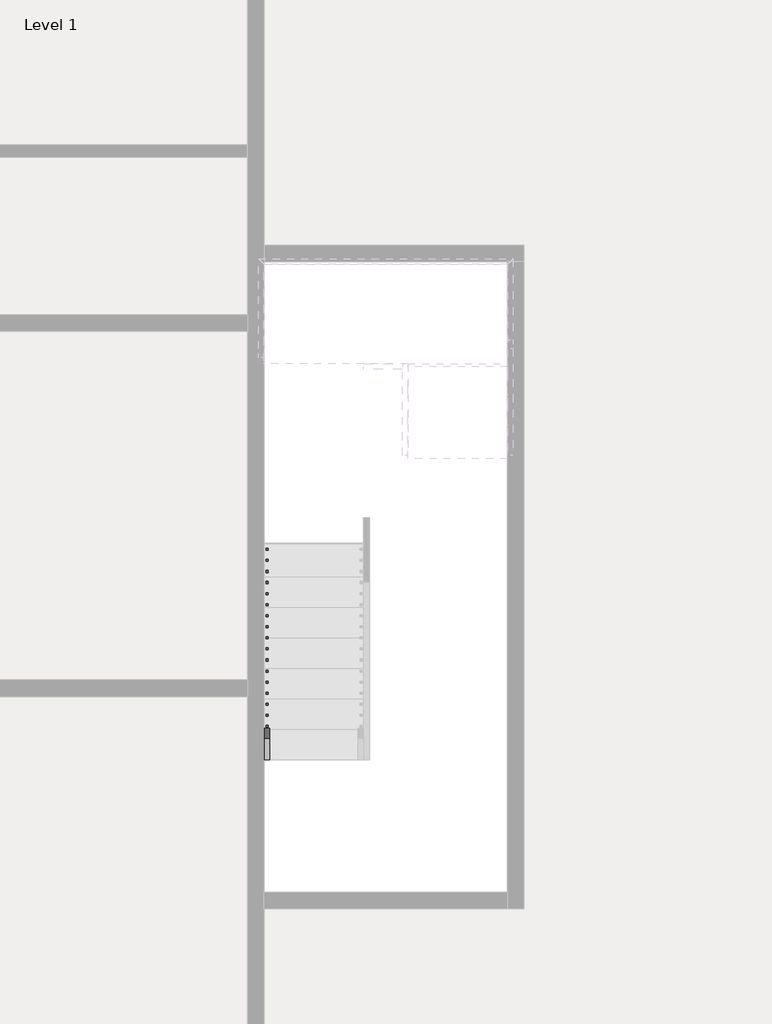
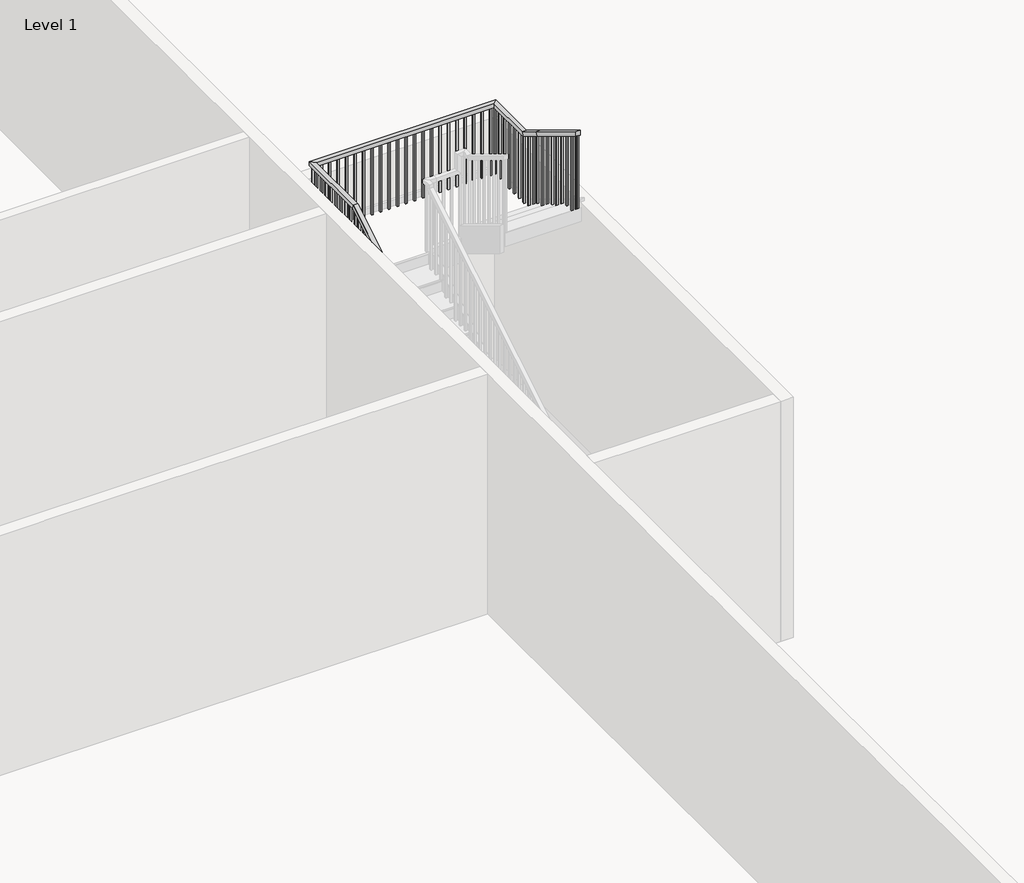
# One storey, part 6 of 8: 1 railing.
"""IFC4 building model written with IfcOpenShell, lengths in millimetres."""

from ifc_helpers import new_model, si_unit, frame, origin, place, context, project, spatial, polyline, outline, extrude, faceted_brep, element, save

model = new_model("IFC4")

# Units and contexts
model_context = context("Model", 3, world=origin())
ifc_project = project(units=[si_unit("LENGTHUNIT", "METRE", prefix="MILLI")], contexts=[model_context])

# Site, building, storey
site = spatial("IfcSite", under=ifc_project)
building = spatial("IfcBuilding", under=site)
storey = spatial("IfcBuildingStorey", under=building, Name="Level 1", Elevation=25234.6172466)

# Railing
placement = place(None, origin())
element("IfcRailing", 1, ObjectType="Handrail - Rectangular", at=placement, inside=storey, context=model_context, shape_type="SolidModel", body=[
    faceted_brep([(-3617.4415084, -23154.3851539, 26318.3505799), (-3617.4415084, -23154.3851539, 26258.9491197), (-3566.6415084, -23154.3851539, 26258.9491197), (-3566.6415084, -23154.3851539, 26318.3505799), (-3617.4415084, -19522.1851539, 28519.6839133), (-3617.4415084, -19507.9927445, 28468.8839133), (-3566.6415084, -19507.9927445, 28468.8839133), (-3566.6415084, -19522.1851539, 28519.6839133), (-3617.4415084, -18607.7851539, 28519.6839133), (-3617.4415084, -18607.7851539, 28468.8839133), (-3566.6415084, -18658.5851539, 28468.8839133), (-3566.6415084, -18658.5851539, 28519.6839133), (-1382.2415084, -18607.7851539, 28519.6839133), (-1382.2415084, -18607.7851539, 28468.8839133), (-1433.0415084, -18658.5851539, 28468.8839133), (-1433.0415084, -18658.5851539, 28519.6839133), (-1382.2415084, -19242.7851539, 28519.6839133), (-1382.2415084, -19256.9775633, 28468.8839133), (-1433.0415084, -19256.9775633, 28468.8839133), (-1433.0415084, -19242.7851539, 28519.6839133), (-1382.2415084, -19522.1851539, 28689.0172466), (-1382.2415084, -19548.5148811, 28645.5731968), (-1433.0415084, -19548.5148811, 28645.5731968), (-1433.0415084, -19522.1851539, 28689.0172466), (-1382.2415084, -20360.3851539, 29197.0172466), (-1433.0415084, -20360.3851539, 29197.0172466), (-1433.0415084, -20360.3851539, 29137.6157863), (-1382.2415084, -20360.3851539, 29137.6157863)], [[[0, 1, 2, 3]], [[1, 0, 4, 5]], [[2, 1, 5, 6]], [[3, 2, 6, 7]], [[0, 3, 7, 4]], [[5, 4, 8, 9]], [[6, 5, 9, 10]], [[7, 6, 10, 11]], [[4, 7, 11, 8]], [[9, 8, 12, 13]], [[10, 9, 13, 14]], [[11, 10, 14, 15]], [[8, 11, 15, 12]], [[13, 12, 16, 17]], [[14, 13, 17, 18]], [[15, 14, 18, 19]], [[12, 15, 19, 16]], [[17, 16, 20, 21]], [[18, 17, 21, 22]], [[19, 18, 22, 23]], [[16, 19, 23, 20]], [[24, 25, 26, 27]], [[21, 20, 24, 27]], [[22, 21, 27, 26]], [[23, 22, 26, 25]], [[20, 23, 25, 24]]]),
    extrude(outline(polyline([(-20325.4601539, 29116.4491197), (-20325.4601539, 28113.2839133), (-20344.5101539, 28113.2839133), (-20344.5101539, 29127.9945742), (-20325.4601539, 29116.4491197)])), frame((-1417.1665084, 0.0, 0.0), z_axis=(1.0, 0.0, 0.0), x_axis=(0.0, 1.0, 0.0)), (0.0, 0.0, 1.0), 19.05),
    extrude(outline(polyline([(-20223.8601539, 29054.8733621), (-20223.8601539, 28113.2839133), (-20242.9101539, 28113.2839133), (-20242.9101539, 29066.4188167), (-20223.8601539, 29054.8733621)])), frame((-1417.1665084, 0.0, 0.0), z_axis=(1.0, 0.0, 0.0), x_axis=(0.0, 1.0, 0.0)), (0.0, 0.0, 1.0), 19.05),
    extrude(outline(polyline([(-20122.2601539, 28993.2976045), (-20122.2601539, 28113.2839133), (-20141.3101539, 28113.2839133), (-20141.3101539, 29004.8430591), (-20122.2601539, 28993.2976045)])), frame((-1417.1665084, 0.0, 0.0), z_axis=(1.0, 0.0, 0.0), x_axis=(0.0, 1.0, 0.0)), (0.0, 0.0, 1.0), 19.05),
    extrude(outline(polyline([(-20020.6601539, 28931.721847), (-20020.6601539, 27943.9505799), (-20039.7101539, 27943.9505799), (-20039.7101539, 28943.2673015), (-20020.6601539, 28931.721847)])), frame((-1417.1665084, 0.0, 0.0), z_axis=(1.0, 0.0, 0.0), x_axis=(0.0, 1.0, 0.0)), (0.0, 0.0, 1.0), 19.05),
    extrude(outline(polyline([(-19919.0601539, 28870.1460894), (-19919.0601539, 27943.9505799), (-19938.1101539, 27943.9505799), (-19938.1101539, 28881.6915439), (-19919.0601539, 28870.1460894)])), frame((-1417.1665084, 0.0, 0.0), z_axis=(1.0, 0.0, 0.0), x_axis=(0.0, 1.0, 0.0)), (0.0, 0.0, 1.0), 19.05),
    extrude(outline(polyline([(-19817.4601539, 28808.5703318), (-19817.4601539, 27943.9505799), (-19836.5101539, 27943.9505799), (-19836.5101539, 28820.1157863), (-19817.4601539, 28808.5703318)])), frame((-1417.1665084, 0.0, 0.0), z_axis=(1.0, 0.0, 0.0), x_axis=(0.0, 1.0, 0.0)), (0.0, 0.0, 1.0), 19.05),
    extrude(outline(polyline([(-19715.8601539, 28746.9945742), (-19715.8601539, 27774.6172466), (-19734.9101539, 27774.6172466), (-19734.9101539, 28758.5400288), (-19715.8601539, 28746.9945742)])), frame((-1417.1665084, 0.0, 0.0), z_axis=(1.0, 0.0, 0.0), x_axis=(0.0, 1.0, 0.0)), (0.0, 0.0, 1.0), 19.05),
    extrude(outline(polyline([(-19614.2601539, 28685.4188167), (-19614.2601539, 27774.6172466), (-19633.3101539, 27774.6172466), (-19633.3101539, 28696.9642712), (-19614.2601539, 28685.4188167)])), frame((-1417.1665084, 0.0, 0.0), z_axis=(1.0, 0.0, 0.0), x_axis=(0.0, 1.0, 0.0)), (0.0, 0.0, 1.0), 19.05),
    extrude(outline(polyline([(-19436.4601539, 28577.6612409), (-19436.4601539, 27605.2839133), (-19455.5101539, 27605.2839133), (-19455.5101539, 28589.2066954), (-19436.4601539, 28577.6612409)])), frame((-1417.1665084, 0.0, 0.0), z_axis=(1.0, 0.0, 0.0), x_axis=(0.0, 1.0, 0.0)), (0.0, 0.0, 1.0), 19.05),
    extrude(outline(polyline([(-19334.8601539, 28516.0854833), (-19334.8601539, 27605.2839133), (-19353.9101539, 27605.2839133), (-19353.9101539, 28527.6309379), (-19334.8601539, 28516.0854833)])), frame((-1417.1665084, 0.0, 0.0), z_axis=(1.0, 0.0, 0.0), x_axis=(0.0, 1.0, 0.0)), (0.0, 0.0, 1.0), 19.05),
    extrude(outline(polyline([(-1398.1165084, -19233.2601539), (-1398.1165084, -19252.3101539), (-1417.1665084, -19252.3101539), (-1417.1665084, -19233.2601539), (-1398.1165084, -19233.2601539)])), frame((0.0, 0.0, 27605.2839133), z_axis=(0.0, 0.0, 1.0), x_axis=(1.0, 0.0, 0.0)), (0.0, 0.0, 1.0), 863.6),
    extrude(outline(polyline([(-1398.1165084, -19131.6601539), (-1398.1165084, -19150.7101539), (-1417.1665084, -19150.7101539), (-1417.1665084, -19131.6601539), (-1398.1165084, -19131.6601539)])), frame((0.0, 0.0, 27605.2839133), z_axis=(0.0, 0.0, 1.0), x_axis=(1.0, 0.0, 0.0)), (0.0, 0.0, 1.0), 863.6),
    extrude(outline(polyline([(-1398.1165084, -19030.0601539), (-1398.1165084, -19049.1101539), (-1417.1665084, -19049.1101539), (-1417.1665084, -19030.0601539), (-1398.1165084, -19030.0601539)])), frame((0.0, 0.0, 27605.2839133), z_axis=(0.0, 0.0, 1.0), x_axis=(1.0, 0.0, 0.0)), (0.0, 0.0, 1.0), 863.6),
    extrude(outline(polyline([(-1398.1165084, -18928.4601539), (-1398.1165084, -18947.5101539), (-1417.1665084, -18947.5101539), (-1417.1665084, -18928.4601539), (-1398.1165084, -18928.4601539)])), frame((0.0, 0.0, 27605.2839133), z_axis=(0.0, 0.0, 1.0), x_axis=(1.0, 0.0, 0.0)), (0.0, 0.0, 1.0), 863.6),
    extrude(outline(polyline([(-1398.1165084, -18826.8601539), (-1398.1165084, -18845.9101539), (-1417.1665084, -18845.9101539), (-1417.1665084, -18826.8601539), (-1398.1165084, -18826.8601539)])), frame((0.0, 0.0, 27605.2839133), z_axis=(0.0, 0.0, 1.0), x_axis=(1.0, 0.0, 0.0)), (0.0, 0.0, 1.0), 863.6),
    extrude(outline(polyline([(-1398.1165084, -18725.2601539), (-1398.1165084, -18744.3101539), (-1417.1665084, -18744.3101539), (-1417.1665084, -18725.2601539), (-1398.1165084, -18725.2601539)])), frame((0.0, 0.0, 27605.2839133), z_axis=(0.0, 0.0, 1.0), x_axis=(1.0, 0.0, 0.0)), (0.0, 0.0, 1.0), 863.6),
    extrude(outline(polyline([(-1467.9665084, -18623.6601539), (-1448.9165084, -18623.6601539), (-1448.9165084, -18642.7101539), (-1467.9665084, -18642.7101539), (-1467.9665084, -18623.6601539)])), frame((0.0, 0.0, 27605.2839133), z_axis=(0.0, 0.0, 1.0), x_axis=(1.0, 0.0, 0.0)), (0.0, 0.0, 1.0), 863.6),
    extrude(outline(polyline([(-1569.5665084, -18623.6601539), (-1550.5165084, -18623.6601539), (-1550.5165084, -18642.7101539), (-1569.5665084, -18642.7101539), (-1569.5665084, -18623.6601539)])), frame((0.0, 0.0, 27605.2839133), z_axis=(0.0, 0.0, 1.0), x_axis=(1.0, 0.0, 0.0)), (0.0, 0.0, 1.0), 863.6),
    extrude(outline(polyline([(-1671.1665084, -18623.6601539), (-1652.1165084, -18623.6601539), (-1652.1165084, -18642.7101539), (-1671.1665084, -18642.7101539), (-1671.1665084, -18623.6601539)])), frame((0.0, 0.0, 27605.2839133), z_axis=(0.0, 0.0, 1.0), x_axis=(1.0, 0.0, 0.0)), (0.0, 0.0, 1.0), 863.6),
    extrude(outline(polyline([(-1772.7665084, -18623.6601539), (-1753.7165084, -18623.6601539), (-1753.7165084, -18642.7101539), (-1772.7665084, -18642.7101539), (-1772.7665084, -18623.6601539)])), frame((0.0, 0.0, 27605.2839133), z_axis=(0.0, 0.0, 1.0), x_axis=(1.0, 0.0, 0.0)), (0.0, 0.0, 1.0), 863.6),
    extrude(outline(polyline([(-1874.3665084, -18623.6601539), (-1855.3165084, -18623.6601539), (-1855.3165084, -18642.7101539), (-1874.3665084, -18642.7101539), (-1874.3665084, -18623.6601539)])), frame((0.0, 0.0, 27605.2839133), z_axis=(0.0, 0.0, 1.0), x_axis=(1.0, 0.0, 0.0)), (0.0, 0.0, 1.0), 863.6),
    extrude(outline(polyline([(-1975.9665084, -18623.6601539), (-1956.9165084, -18623.6601539), (-1956.9165084, -18642.7101539), (-1975.9665084, -18642.7101539), (-1975.9665084, -18623.6601539)])), frame((0.0, 0.0, 27605.2839133), z_axis=(0.0, 0.0, 1.0), x_axis=(1.0, 0.0, 0.0)), (0.0, 0.0, 1.0), 863.6),
    extrude(outline(polyline([(-2077.5665084, -18623.6601539), (-2058.5165084, -18623.6601539), (-2058.5165084, -18642.7101539), (-2077.5665084, -18642.7101539), (-2077.5665084, -18623.6601539)])), frame((0.0, 0.0, 27605.2839133), z_axis=(0.0, 0.0, 1.0), x_axis=(1.0, 0.0, 0.0)), (0.0, 0.0, 1.0), 863.6),
    extrude(outline(polyline([(-2179.1665084, -18623.6601539), (-2160.1165084, -18623.6601539), (-2160.1165084, -18642.7101539), (-2179.1665084, -18642.7101539), (-2179.1665084, -18623.6601539)])), frame((0.0, 0.0, 27605.2839133), z_axis=(0.0, 0.0, 1.0), x_axis=(1.0, 0.0, 0.0)), (0.0, 0.0, 1.0), 863.6),
    extrude(outline(polyline([(-2280.7665084, -18623.6601539), (-2261.7165084, -18623.6601539), (-2261.7165084, -18642.7101539), (-2280.7665084, -18642.7101539), (-2280.7665084, -18623.6601539)])), frame((0.0, 0.0, 27605.2839133), z_axis=(0.0, 0.0, 1.0), x_axis=(1.0, 0.0, 0.0)), (0.0, 0.0, 1.0), 863.6),
    extrude(outline(polyline([(-2382.3665084, -18623.6601539), (-2363.3165084, -18623.6601539), (-2363.3165084, -18642.7101539), (-2382.3665084, -18642.7101539), (-2382.3665084, -18623.6601539)])), frame((0.0, 0.0, 27605.2839133), z_axis=(0.0, 0.0, 1.0), x_axis=(1.0, 0.0, 0.0)), (0.0, 0.0, 1.0), 863.6),
    extrude(outline(polyline([(-2483.9665084, -18623.6601539), (-2464.9165084, -18623.6601539), (-2464.9165084, -18642.7101539), (-2483.9665084, -18642.7101539), (-2483.9665084, -18623.6601539)])), frame((0.0, 0.0, 27605.2839133), z_axis=(0.0, 0.0, 1.0), x_axis=(1.0, 0.0, 0.0)), (0.0, 0.0, 1.0), 863.6),
    extrude(outline(polyline([(-2585.5665084, -18623.6601539), (-2566.5165084, -18623.6601539), (-2566.5165084, -18642.7101539), (-2585.5665084, -18642.7101539), (-2585.5665084, -18623.6601539)])), frame((0.0, 0.0, 27605.2839133), z_axis=(0.0, 0.0, 1.0), x_axis=(1.0, 0.0, 0.0)), (0.0, 0.0, 1.0), 863.6),
    extrude(outline(polyline([(-2687.1665084, -18623.6601539), (-2668.1165084, -18623.6601539), (-2668.1165084, -18642.7101539), (-2687.1665084, -18642.7101539), (-2687.1665084, -18623.6601539)])), frame((0.0, 0.0, 27605.2839133), z_axis=(0.0, 0.0, 1.0), x_axis=(1.0, 0.0, 0.0)), (0.0, 0.0, 1.0), 863.6),
    extrude(outline(polyline([(-2788.7665084, -18623.6601539), (-2769.7165084, -18623.6601539), (-2769.7165084, -18642.7101539), (-2788.7665084, -18642.7101539), (-2788.7665084, -18623.6601539)])), frame((0.0, 0.0, 27605.2839133), z_axis=(0.0, 0.0, 1.0), x_axis=(1.0, 0.0, 0.0)), (0.0, 0.0, 1.0), 863.6),
    extrude(outline(polyline([(-2890.3665084, -18623.6601539), (-2871.3165084, -18623.6601539), (-2871.3165084, -18642.7101539), (-2890.3665084, -18642.7101539), (-2890.3665084, -18623.6601539)])), frame((0.0, 0.0, 27605.2839133), z_axis=(0.0, 0.0, 1.0), x_axis=(1.0, 0.0, 0.0)), (0.0, 0.0, 1.0), 863.6),
    extrude(outline(polyline([(-2991.9665084, -18623.6601539), (-2972.9165084, -18623.6601539), (-2972.9165084, -18642.7101539), (-2991.9665084, -18642.7101539), (-2991.9665084, -18623.6601539)])), frame((0.0, 0.0, 27605.2839133), z_axis=(0.0, 0.0, 1.0), x_axis=(1.0, 0.0, 0.0)), (0.0, 0.0, 1.0), 863.6),
    extrude(outline(polyline([(-3093.5665084, -18623.6601539), (-3074.5165084, -18623.6601539), (-3074.5165084, -18642.7101539), (-3093.5665084, -18642.7101539), (-3093.5665084, -18623.6601539)])), frame((0.0, 0.0, 27605.2839133), z_axis=(0.0, 0.0, 1.0), x_axis=(1.0, 0.0, 0.0)), (0.0, 0.0, 1.0), 863.6),
    extrude(outline(polyline([(-3195.1665084, -18623.6601539), (-3176.1165084, -18623.6601539), (-3176.1165084, -18642.7101539), (-3195.1665084, -18642.7101539), (-3195.1665084, -18623.6601539)])), frame((0.0, 0.0, 27605.2839133), z_axis=(0.0, 0.0, 1.0), x_axis=(1.0, 0.0, 0.0)), (0.0, 0.0, 1.0), 863.6),
    extrude(outline(polyline([(-3296.7665084, -18623.6601539), (-3277.7165084, -18623.6601539), (-3277.7165084, -18642.7101539), (-3296.7665084, -18642.7101539), (-3296.7665084, -18623.6601539)])), frame((0.0, 0.0, 27605.2839133), z_axis=(0.0, 0.0, 1.0), x_axis=(1.0, 0.0, 0.0)), (0.0, 0.0, 1.0), 863.6),
    extrude(outline(polyline([(-3398.3665084, -18623.6601539), (-3379.3165084, -18623.6601539), (-3379.3165084, -18642.7101539), (-3398.3665084, -18642.7101539), (-3398.3665084, -18623.6601539)])), frame((0.0, 0.0, 27605.2839133), z_axis=(0.0, 0.0, 1.0), x_axis=(1.0, 0.0, 0.0)), (0.0, 0.0, 1.0), 863.6),
    extrude(outline(polyline([(-3499.9665084, -18623.6601539), (-3480.9165084, -18623.6601539), (-3480.9165084, -18642.7101539), (-3499.9665084, -18642.7101539), (-3499.9665084, -18623.6601539)])), frame((0.0, 0.0, 27605.2839133), z_axis=(0.0, 0.0, 1.0), x_axis=(1.0, 0.0, 0.0)), (0.0, 0.0, 1.0), 863.6),
    extrude(outline(polyline([(-3601.5665084, -18718.9101539), (-3601.5665084, -18699.8601539), (-3582.5165084, -18699.8601539), (-3582.5165084, -18718.9101539), (-3601.5665084, -18718.9101539)])), frame((0.0, 0.0, 27605.2839133), z_axis=(0.0, 0.0, 1.0), x_axis=(1.0, 0.0, 0.0)), (0.0, 0.0, 1.0), 863.6),
    extrude(outline(polyline([(-3601.5665084, -18820.5101539), (-3601.5665084, -18801.4601539), (-3582.5165084, -18801.4601539), (-3582.5165084, -18820.5101539), (-3601.5665084, -18820.5101539)])), frame((0.0, 0.0, 27605.2839133), z_axis=(0.0, 0.0, 1.0), x_axis=(1.0, 0.0, 0.0)), (0.0, 0.0, 1.0), 863.6),
    extrude(outline(polyline([(-3601.5665084, -18922.1101539), (-3601.5665084, -18903.0601539), (-3582.5165084, -18903.0601539), (-3582.5165084, -18922.1101539), (-3601.5665084, -18922.1101539)])), frame((0.0, 0.0, 27605.2839133), z_axis=(0.0, 0.0, 1.0), x_axis=(1.0, 0.0, 0.0)), (0.0, 0.0, 1.0), 863.6),
    extrude(outline(polyline([(-3601.5665084, -19023.7101539), (-3601.5665084, -19004.6601539), (-3582.5165084, -19004.6601539), (-3582.5165084, -19023.7101539), (-3601.5665084, -19023.7101539)])), frame((0.0, 0.0, 27605.2839133), z_axis=(0.0, 0.0, 1.0), x_axis=(1.0, 0.0, 0.0)), (0.0, 0.0, 1.0), 863.6),
    extrude(outline(polyline([(-3601.5665084, -19125.3101539), (-3601.5665084, -19106.2601539), (-3582.5165084, -19106.2601539), (-3582.5165084, -19125.3101539), (-3601.5665084, -19125.3101539)])), frame((0.0, 0.0, 27605.2839133), z_axis=(0.0, 0.0, 1.0), x_axis=(1.0, 0.0, 0.0)), (0.0, 0.0, 1.0), 863.6),
    extrude(outline(polyline([(-3601.5665084, -19226.9101539), (-3601.5665084, -19207.8601539), (-3582.5165084, -19207.8601539), (-3582.5165084, -19226.9101539), (-3601.5665084, -19226.9101539)])), frame((0.0, 0.0, 27605.2839133), z_axis=(0.0, 0.0, 1.0), x_axis=(1.0, 0.0, 0.0)), (0.0, 0.0, 1.0), 863.6),
    extrude(outline(polyline([(-3601.5665084, -19328.5101539), (-3601.5665084, -19309.4601539), (-3582.5165084, -19309.4601539), (-3582.5165084, -19328.5101539), (-3601.5665084, -19328.5101539)])), frame((0.0, 0.0, 27605.2839133), z_axis=(0.0, 0.0, 1.0), x_axis=(1.0, 0.0, 0.0)), (0.0, 0.0, 1.0), 863.6),
    extrude(outline(polyline([(-3601.5665084, -19430.1101539), (-3601.5665084, -19411.0601539), (-3582.5165084, -19411.0601539), (-3582.5165084, -19430.1101539), (-3601.5665084, -19430.1101539)])), frame((0.0, 0.0, 27605.2839133), z_axis=(0.0, 0.0, 1.0), x_axis=(1.0, 0.0, 0.0)), (0.0, 0.0, 1.0), 863.6),
    extrude(outline(polyline([(-19588.8601539, 28419.8733621), (-19588.8601539, 27435.9505799), (-19607.9101539, 27435.9505799), (-19607.9101539, 28408.3279076), (-19588.8601539, 28419.8733621)])), frame((-3601.5665084, 0.0, 0.0), z_axis=(1.0, 0.0, 0.0), x_axis=(0.0, 1.0, 0.0)), (0.0, 0.0, 1.0), 19.05),
    extrude(outline(polyline([(-19690.4601539, 28358.2976045), (-19690.4601539, 27435.9505799), (-19709.5101539, 27435.9505799), (-19709.5101539, 28346.75215), (-19690.4601539, 28358.2976045)])), frame((-3601.5665084, 0.0, 0.0), z_axis=(1.0, 0.0, 0.0), x_axis=(0.0, 1.0, 0.0)), (0.0, 0.0, 1.0), 19.05),
    extrude(outline(polyline([(-19792.0601539, 28296.721847), (-19792.0601539, 27435.9505799), (-19811.1101539, 27435.9505799), (-19811.1101539, 28285.1763924), (-19792.0601539, 28296.721847)])), frame((-3601.5665084, 0.0, 0.0), z_axis=(1.0, 0.0, 0.0), x_axis=(0.0, 1.0, 0.0)), (0.0, 0.0, 1.0), 19.05),
    extrude(outline(polyline([(-19893.6601539, 28235.1460894), (-19893.6601539, 27266.6172466), (-19912.7101539, 27266.6172466), (-19912.7101539, 28223.6006348), (-19893.6601539, 28235.1460894)])), frame((-3601.5665084, 0.0, 0.0), z_axis=(1.0, 0.0, 0.0), x_axis=(0.0, 1.0, 0.0)), (0.0, 0.0, 1.0), 19.05),
    extrude(outline(polyline([(-19995.2601539, 28173.5703318), (-19995.2601539, 27266.6172466), (-20014.3101539, 27266.6172466), (-20014.3101539, 28162.0248773), (-19995.2601539, 28173.5703318)])), frame((-3601.5665084, 0.0, 0.0), z_axis=(1.0, 0.0, 0.0), x_axis=(0.0, 1.0, 0.0)), (0.0, 0.0, 1.0), 19.05),
    extrude(outline(polyline([(-20096.8601539, 28111.9945742), (-20096.8601539, 27097.2839133), (-20115.9101539, 27097.2839133), (-20115.9101539, 28100.4491197), (-20096.8601539, 28111.9945742)])), frame((-3601.5665084, 0.0, 0.0), z_axis=(1.0, 0.0, 0.0), x_axis=(0.0, 1.0, 0.0)), (0.0, 0.0, 1.0), 19.05),
    extrude(outline(polyline([(-20198.4601539, 28050.4188167), (-20198.4601539, 27097.2839133), (-20217.5101539, 27097.2839133), (-20217.5101539, 28038.8733621), (-20198.4601539, 28050.4188167)])), frame((-3601.5665084, 0.0, 0.0), z_axis=(1.0, 0.0, 0.0), x_axis=(0.0, 1.0, 0.0)), (0.0, 0.0, 1.0), 19.05),
    extrude(outline(polyline([(-20300.0601539, 27988.8430591), (-20300.0601539, 27097.2839133), (-20319.1101539, 27097.2839133), (-20319.1101539, 27977.2976045), (-20300.0601539, 27988.8430591)])), frame((-3601.5665084, 0.0, 0.0), z_axis=(1.0, 0.0, 0.0), x_axis=(0.0, 1.0, 0.0)), (0.0, 0.0, 1.0), 19.05),
    extrude(outline(polyline([(-20401.6601539, 27927.2673015), (-20401.6601539, 26927.9505799), (-20420.7101539, 26927.9505799), (-20420.7101539, 27915.721847), (-20401.6601539, 27927.2673015)])), frame((-3601.5665084, 0.0, 0.0), z_axis=(1.0, 0.0, 0.0), x_axis=(0.0, 1.0, 0.0)), (0.0, 0.0, 1.0), 19.05),
    extrude(outline(polyline([(-20503.2601539, 27865.6915439), (-20503.2601539, 26927.9505799), (-20522.3101539, 26927.9505799), (-20522.3101539, 27854.1460894), (-20503.2601539, 27865.6915439)])), frame((-3601.5665084, 0.0, 0.0), z_axis=(1.0, 0.0, 0.0), x_axis=(0.0, 1.0, 0.0)), (0.0, 0.0, 1.0), 19.05),
    extrude(outline(polyline([(-20604.8601539, 27804.1157863), (-20604.8601539, 26927.9505799), (-20623.9101539, 26927.9505799), (-20623.9101539, 27792.5703318), (-20604.8601539, 27804.1157863)])), frame((-3601.5665084, 0.0, 0.0), z_axis=(1.0, 0.0, 0.0), x_axis=(0.0, 1.0, 0.0)), (0.0, 0.0, 1.0), 19.05),
    extrude(outline(polyline([(-20706.4601539, 27742.5400288), (-20706.4601539, 26758.6172466), (-20725.5101539, 26758.6172466), (-20725.5101539, 27730.9945742), (-20706.4601539, 27742.5400288)])), frame((-3601.5665084, 0.0, 0.0), z_axis=(1.0, 0.0, 0.0), x_axis=(0.0, 1.0, 0.0)), (0.0, 0.0, 1.0), 19.05),
    extrude(outline(polyline([(-20808.0601539, 27680.9642712), (-20808.0601539, 26758.6172466), (-20827.1101539, 26758.6172466), (-20827.1101539, 27669.4188167), (-20808.0601539, 27680.9642712)])), frame((-3601.5665084, 0.0, 0.0), z_axis=(1.0, 0.0, 0.0), x_axis=(0.0, 1.0, 0.0)), (0.0, 0.0, 1.0), 19.05),
    extrude(outline(polyline([(-20909.6601539, 27619.3885136), (-20909.6601539, 26758.6172466), (-20928.7101539, 26758.6172466), (-20928.7101539, 27607.8430591), (-20909.6601539, 27619.3885136)])), frame((-3601.5665084, 0.0, 0.0), z_axis=(1.0, 0.0, 0.0), x_axis=(0.0, 1.0, 0.0)), (0.0, 0.0, 1.0), 19.05),
    extrude(outline(polyline([(-21011.2601539, 27557.812756), (-21011.2601539, 26589.2839133), (-21030.3101539, 26589.2839133), (-21030.3101539, 27546.2673015), (-21011.2601539, 27557.812756)])), frame((-3601.5665084, 0.0, 0.0), z_axis=(1.0, 0.0, 0.0), x_axis=(0.0, 1.0, 0.0)), (0.0, 0.0, 1.0), 19.05),
    extrude(outline(polyline([(-21112.8601539, 27496.2369985), (-21112.8601539, 26589.2839133), (-21131.9101539, 26589.2839133), (-21131.9101539, 27484.6915439), (-21112.8601539, 27496.2369985)])), frame((-3601.5665084, 0.0, 0.0), z_axis=(1.0, 0.0, 0.0), x_axis=(0.0, 1.0, 0.0)), (0.0, 0.0, 1.0), 19.05),
    extrude(outline(polyline([(-21214.4601539, 27434.6612409), (-21214.4601539, 26419.9505799), (-21233.5101539, 26419.9505799), (-21233.5101539, 27423.1157863), (-21214.4601539, 27434.6612409)])), frame((-3601.5665084, 0.0, 0.0), z_axis=(1.0, 0.0, 0.0), x_axis=(0.0, 1.0, 0.0)), (0.0, 0.0, 1.0), 19.05),
    extrude(outline(polyline([(-21316.0601539, 27373.0854833), (-21316.0601539, 26419.9505799), (-21335.1101539, 26419.9505799), (-21335.1101539, 27361.5400288), (-21316.0601539, 27373.0854833)])), frame((-3601.5665084, 0.0, 0.0), z_axis=(1.0, 0.0, 0.0), x_axis=(0.0, 1.0, 0.0)), (0.0, 0.0, 1.0), 19.05),
    extrude(outline(polyline([(-21417.6601539, 27311.5097257), (-21417.6601539, 26419.9505799), (-21436.7101539, 26419.9505799), (-21436.7101539, 27299.9642712), (-21417.6601539, 27311.5097257)])), frame((-3601.5665084, 0.0, 0.0), z_axis=(1.0, 0.0, 0.0), x_axis=(0.0, 1.0, 0.0)), (0.0, 0.0, 1.0), 19.05),
    extrude(outline(polyline([(-21519.2601539, 27249.9339682), (-21519.2601539, 26250.6172466), (-21538.3101539, 26250.6172466), (-21538.3101539, 27238.3885136), (-21519.2601539, 27249.9339682)])), frame((-3601.5665084, 0.0, 0.0), z_axis=(1.0, 0.0, 0.0), x_axis=(0.0, 1.0, 0.0)), (0.0, 0.0, 1.0), 19.05),
    extrude(outline(polyline([(-21620.8601539, 27188.3582106), (-21620.8601539, 26250.6172466), (-21639.9101539, 26250.6172466), (-21639.9101539, 27176.812756), (-21620.8601539, 27188.3582106)])), frame((-3601.5665084, 0.0, 0.0), z_axis=(1.0, 0.0, 0.0), x_axis=(0.0, 1.0, 0.0)), (0.0, 0.0, 1.0), 19.05),
    extrude(outline(polyline([(-21722.4601539, 27126.782453), (-21722.4601539, 26250.6172466), (-21741.5101539, 26250.6172466), (-21741.5101539, 27115.2369985), (-21722.4601539, 27126.782453)])), frame((-3601.5665084, 0.0, 0.0), z_axis=(1.0, 0.0, 0.0), x_axis=(0.0, 1.0, 0.0)), (0.0, 0.0, 1.0), 19.05),
    extrude(outline(polyline([(-21824.0601539, 27065.2066954), (-21824.0601539, 26081.2839133), (-21843.1101539, 26081.2839133), (-21843.1101539, 27053.6612409), (-21824.0601539, 27065.2066954)])), frame((-3601.5665084, 0.0, 0.0), z_axis=(1.0, 0.0, 0.0), x_axis=(0.0, 1.0, 0.0)), (0.0, 0.0, 1.0), 19.05),
    extrude(outline(polyline([(-21925.6601539, 27003.6309379), (-21925.6601539, 26081.2839133), (-21944.7101539, 26081.2839133), (-21944.7101539, 26992.0854833), (-21925.6601539, 27003.6309379)])), frame((-3601.5665084, 0.0, 0.0), z_axis=(1.0, 0.0, 0.0), x_axis=(0.0, 1.0, 0.0)), (0.0, 0.0, 1.0), 19.05),
    extrude(outline(polyline([(-22027.2601539, 26942.0551803), (-22027.2601539, 26081.2839133), (-22046.3101539, 26081.2839133), (-22046.3101539, 26930.5097257), (-22027.2601539, 26942.0551803)])), frame((-3601.5665084, 0.0, 0.0), z_axis=(1.0, 0.0, 0.0), x_axis=(0.0, 1.0, 0.0)), (0.0, 0.0, 1.0), 19.05),
    extrude(outline(polyline([(-22128.8601539, 26880.4794227), (-22128.8601539, 25911.9505799), (-22147.9101539, 25911.9505799), (-22147.9101539, 26868.9339682), (-22128.8601539, 26880.4794227)])), frame((-3601.5665084, 0.0, 0.0), z_axis=(1.0, 0.0, 0.0), x_axis=(0.0, 1.0, 0.0)), (0.0, 0.0, 1.0), 19.05),
    extrude(outline(polyline([(-22230.4601539, 26818.9036651), (-22230.4601539, 25911.9505799), (-22249.5101539, 25911.9505799), (-22249.5101539, 26807.3582106), (-22230.4601539, 26818.9036651)])), frame((-3601.5665084, 0.0, 0.0), z_axis=(1.0, 0.0, 0.0), x_axis=(0.0, 1.0, 0.0)), (0.0, 0.0, 1.0), 19.05),
    extrude(outline(polyline([(-22332.0601539, 26757.3279076), (-22332.0601539, 25742.6172466), (-22351.1101539, 25742.6172466), (-22351.1101539, 26745.782453), (-22332.0601539, 26757.3279076)])), frame((-3601.5665084, 0.0, 0.0), z_axis=(1.0, 0.0, 0.0), x_axis=(0.0, 1.0, 0.0)), (0.0, 0.0, 1.0), 19.05),
    extrude(outline(polyline([(-22433.6601539, 26695.75215), (-22433.6601539, 25742.6172466), (-22452.7101539, 25742.6172466), (-22452.7101539, 26684.2066954), (-22433.6601539, 26695.75215)])), frame((-3601.5665084, 0.0, 0.0), z_axis=(1.0, 0.0, 0.0), x_axis=(0.0, 1.0, 0.0)), (0.0, 0.0, 1.0), 19.05),
    extrude(outline(polyline([(-22535.2601539, 26634.1763924), (-22535.2601539, 25742.6172466), (-22554.3101539, 25742.6172466), (-22554.3101539, 26622.6309379), (-22535.2601539, 26634.1763924)])), frame((-3601.5665084, 0.0, 0.0), z_axis=(1.0, 0.0, 0.0), x_axis=(0.0, 1.0, 0.0)), (0.0, 0.0, 1.0), 19.05),
    extrude(outline(polyline([(-22636.8601539, 26572.6006348), (-22636.8601539, 25573.2839133), (-22655.9101539, 25573.2839133), (-22655.9101539, 26561.0551803), (-22636.8601539, 26572.6006348)])), frame((-3601.5665084, 0.0, 0.0), z_axis=(1.0, 0.0, 0.0), x_axis=(0.0, 1.0, 0.0)), (0.0, 0.0, 1.0), 19.05),
    extrude(outline(polyline([(-22738.4601539, 26511.0248773), (-22738.4601539, 25573.2839133), (-22757.5101539, 25573.2839133), (-22757.5101539, 26499.4794227), (-22738.4601539, 26511.0248773)])), frame((-3601.5665084, 0.0, 0.0), z_axis=(1.0, 0.0, 0.0), x_axis=(0.0, 1.0, 0.0)), (0.0, 0.0, 1.0), 19.05),
    extrude(outline(polyline([(-22840.0601539, 26449.4491197), (-22840.0601539, 25573.2839133), (-22859.1101539, 25573.2839133), (-22859.1101539, 26437.9036651), (-22840.0601539, 26449.4491197)])), frame((-3601.5665084, 0.0, 0.0), z_axis=(1.0, 0.0, 0.0), x_axis=(0.0, 1.0, 0.0)), (0.0, 0.0, 1.0), 19.05),
    extrude(outline(polyline([(-22941.6601539, 26387.8733621), (-22941.6601539, 25403.9505799), (-22960.7101539, 25403.9505799), (-22960.7101539, 26376.3279076), (-22941.6601539, 26387.8733621)])), frame((-3601.5665084, 0.0, 0.0), z_axis=(1.0, 0.0, 0.0), x_axis=(0.0, 1.0, 0.0)), (0.0, 0.0, 1.0), 19.05),
    extrude(outline(polyline([(-23043.2601539, 26326.2976045), (-23043.2601539, 25403.9505799), (-23062.3101539, 25403.9505799), (-23062.3101539, 26314.75215), (-23043.2601539, 26326.2976045)])), frame((-3601.5665084, 0.0, 0.0), z_axis=(1.0, 0.0, 0.0), x_axis=(0.0, 1.0, 0.0)), (0.0, 0.0, 1.0), 19.05),
    extrude(outline(polyline([(-19512.6601539, 28623.8430591), (-19512.6601539, 27605.2839133), (-19531.7101539, 27605.2839133), (-19531.7101539, 28635.3885136), (-19512.6601539, 28623.8430591)])), frame((-1417.1665084, 0.0, 0.0), z_axis=(1.0, 0.0, 0.0), x_axis=(0.0, 1.0, 0.0)), (0.0, 0.0, 1.0), 19.05),
    extrude(outline(polyline([(-1417.1665084, -18623.6601539), (-1398.1165084, -18623.6601539), (-1398.1165084, -18642.7101539), (-1417.1665084, -18642.7101539), (-1417.1665084, -18623.6601539)])), frame((0.0, 0.0, 27605.2839133), z_axis=(0.0, 0.0, 1.0), x_axis=(1.0, 0.0, 0.0)), (0.0, 0.0, 1.0), 863.6),
    extrude(outline(polyline([(-3601.5665084, -18642.7101539), (-3601.5665084, -18623.6601539), (-3582.5165084, -18623.6601539), (-3582.5165084, -18642.7101539), (-3601.5665084, -18642.7101539)])), frame((0.0, 0.0, 27605.2839133), z_axis=(0.0, 0.0, 1.0), x_axis=(1.0, 0.0, 0.0)), (0.0, 0.0, 1.0), 863.6),
    extrude(outline(polyline([(-19512.6601539, 28466.0551803), (-19512.6601539, 27605.2839133), (-19531.7101539, 27605.2839133), (-19531.7101539, 28454.5097257), (-19512.6601539, 28466.0551803)])), frame((-3601.5665084, 0.0, 0.0), z_axis=(1.0, 0.0, 0.0), x_axis=(0.0, 1.0, 0.0)), (0.0, 0.0, 1.0), 19.05),
    extrude(outline(polyline([(-20341.3351539, 29126.0703318), (-20341.3351539, 28113.2839133), (-20360.3851539, 28113.2839133), (-20360.3851539, 29137.6157863), (-20341.3351539, 29126.0703318)])), frame((-1417.1665084, 0.0, 0.0), z_axis=(1.0, 0.0, 0.0), x_axis=(0.0, 1.0, 0.0)), (0.0, 0.0, 1.0), 19.05),
    extrude(outline(polyline([(-23135.3351539, 26270.4945742), (-23135.3351539, 25403.9505799), (-23154.3851539, 25403.9505799), (-23154.3851539, 26258.9491197), (-23135.3351539, 26270.4945742)])), frame((-3601.5665084, 0.0, 0.0), z_axis=(1.0, 0.0, 0.0), x_axis=(0.0, 1.0, 0.0)), (0.0, 0.0, 1.0), 19.05),
])

save(model, "model.ifc")

# Revit data of these elements
# Type "Handrail - Rectangular"
#   Assembly Code = "C2010400"
#   built-in parameter 1008612 = 0.0416667 (stored number, unit not read)
#   built-in parameter 1008611 = 0.0416667 (stored number, unit not read)
#   built-in parameter 1008609 = 0.333333 (stored number, unit not read)
#   built-in parameter 1008604 = 0.166667 (stored number, unit not read)
#   built-in parameter 1008603 = 0.166667 (stored number, unit not read)
#   Railing Height = 3' - 0"
#   built-in parameter 1008630 = 2
#   built-in parameter 1008610 = 2
#   built-in parameter 1008618 = Baluster - Square : 3/4"
# Element 1 (IfcRailing, "Handrail - Rectangular")
#   Phase Created = New Construction
